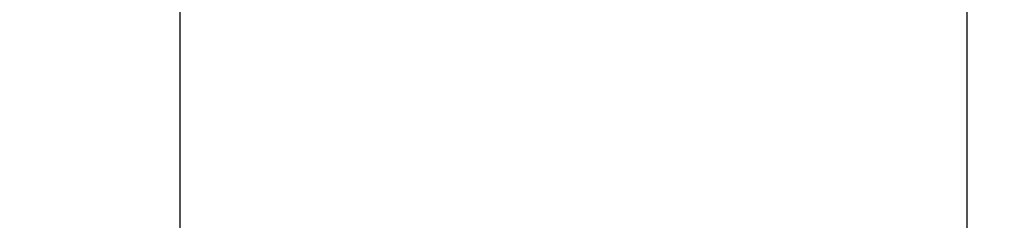
# Model space of a CAD drawing. Units: inches. Extents: x 2091 to 2899, y 967 to 2217.
# Tile 21 of 256: x 2351 to 2390, y 1080 to 1088. Entities that reach past the tile are written whole.
import ezdxf

# ---------------------------------------------------------------- set-up
doc = ezdxf.new("R2010")
doc.units = ezdxf.units.IN
doc.layers.add('A-ANNO-DIMS', color=2, linetype='Continuous', lineweight=18)
doc.styles.get("Standard").update_dxf_attribs({"font": 'arial.ttf'})
doc.dimstyles.new('ISO-25', dxfattribs={"dimtxt": 4, "dimasz": 4, "dimexe": 1.25, "dimexo": 0.625, "dimtad": 1, "dimdec": 0, "dimlunit": 3, "dimtxsty": 'Standard', "dimcen": 2.5, "dimadec": 0, "dimazin": 0, "dimtfac": 1, "dimtdec": 0, "dimtmove": 0, "dimatfit": 3, "dimfxl": 1, "dimarcsym": 0})

# ---------------------------------------------------------------- blocks, each defined once
blk = doc.blocks.new('*D68')
at = {"layer": 'A-ANNO-DIMS', "color": 0, "lineweight": -2, "transparency": 16777216}
for p, q in [((2317.144, 1535.794), (2317.144, 969.464)), ((2459.384, 1535.794), (2459.384, 969.464)), ((2321.144, 970.714), (2455.384, 970.714))]:
    blk.add_line(p, q, dxfattribs=at)
at = {"layer": 'A-ANNO-DIMS', "color": 0, "transparency": 16777216}
for points in [[(2321.144, 971.381), (2321.144, 970.048), (2317.144, 970.714)], [(2455.384, 971.381), (2455.384, 970.048), (2459.384, 970.714)]]:
    blk.add_solid(points, dxfattribs=at)
at = {"layer": 'Defpoints', "color": 0, "transparency": 16777216}
for p in [(2317.144, 1536.419), (2459.384, 1536.419), (2459.384, 970.714)]:
    blk.add_point(p, dxfattribs=at)
at = {"layer": 'A-ANNO-DIMS', "color": 0, "transparency": 16777216, "insert": (2388.264, 973.382), "char_height": 4, "attachment_point": 5}
blk.add_mtext('11\'-10"', dxfattribs=at)
blk = doc.blocks.new('*D71')
at = {"layer": 'A-ANNO-DIMS', "color": 0, "lineweight": -2, "transparency": 16777216}
for p, q in [((2212.144, 1351.294), (2212.144, 969.464)), ((2452.144, 1351.294), (2452.144, 969.464)), ((2216.144, 970.714), (2448.144, 970.714))]:
    blk.add_line(p, q, dxfattribs=at)
at = {"layer": 'A-ANNO-DIMS', "color": 0, "transparency": 16777216}
for points in [[(2216.144, 971.381), (2216.144, 970.048), (2212.144, 970.714)], [(2448.144, 971.381), (2448.144, 970.048), (2452.144, 970.714)]]:
    blk.add_solid(points, dxfattribs=at)
at = {"layer": 'Defpoints', "color": 0, "transparency": 16777216}
for p in [(2212.144, 1351.919), (2452.144, 1351.919), (2452.144, 970.714)]:
    blk.add_point(p, dxfattribs=at)
at = {"layer": 'A-ANNO-DIMS', "color": 0, "transparency": 16777216, "insert": (2332.144, 973.382), "char_height": 4, "attachment_point": 5}
blk.add_mtext('20\'-0"', dxfattribs=at)
blk = doc.blocks.new('*D82')
at = {"layer": 'A-ANNO-DIMS', "color": 0, "lineweight": -2, "transparency": 16777216}
for p, q in [((2357.434, 1549.361), (2357.434, 969.464)), ((2388.969, 1549.361), (2388.969, 969.464)), ((2361.434, 970.714), (2384.969, 970.714))]:
    blk.add_line(p, q, dxfattribs=at)
at = {"layer": 'A-ANNO-DIMS', "color": 0, "transparency": 16777216}
for points in [[(2361.434, 971.381), (2361.434, 970.048), (2357.434, 970.714)], [(2384.969, 971.381), (2384.969, 970.048), (2388.969, 970.714)]]:
    blk.add_solid(points, dxfattribs=at)
at = {"layer": 'Defpoints', "color": 0, "transparency": 16777216}
for p in [(2357.434, 1549.986), (2388.969, 1549.986), (2388.969, 970.714)]:
    blk.add_point(p, dxfattribs=at)
at = {"layer": 'A-ANNO-DIMS', "color": 0, "transparency": 16777216, "insert": (2373.202, 973.408), "char_height": 4, "attachment_point": 5}
blk.add_mtext('2\'-7 1/2"', dxfattribs=at)

msp = doc.modelspace()

# ---------------------------------------------------------------- dimensions: what is measured, and where the dimension line sits
at = {"layer": 'A-ANNO-DIMS'}
for base, p1, p2, picture, middle in [((2388.969, 970.714), (2357.434, 1549.986), (2388.969, 1549.986), '*D82', (2373.202, 973.408)), ((2459.384, 970.714), (2317.144, 1536.419), (2459.384, 1536.419), '*D68', (2388.264, 973.382)), ((2452.144, 970.714), (2212.144, 1351.919), (2452.144, 1351.919), '*D71', (2332.144, 973.382))]:
    dim = msp.add_linear_dim(base=base, p1=p1, p2=p2, dimstyle='ISO-25', override={"dimdec": 1, "dimlfac": 1, "dimrnd": 0, "dimzin": 1, "dimdsep": 46, "dimlunit": 4, "dimfrac": 2}, dxfattribs=at)
    dim.commit()
    dim.dimension.update_dxf_attribs({"geometry": picture, "text_midpoint": middle})

doc.saveas('drawing.dxf')
